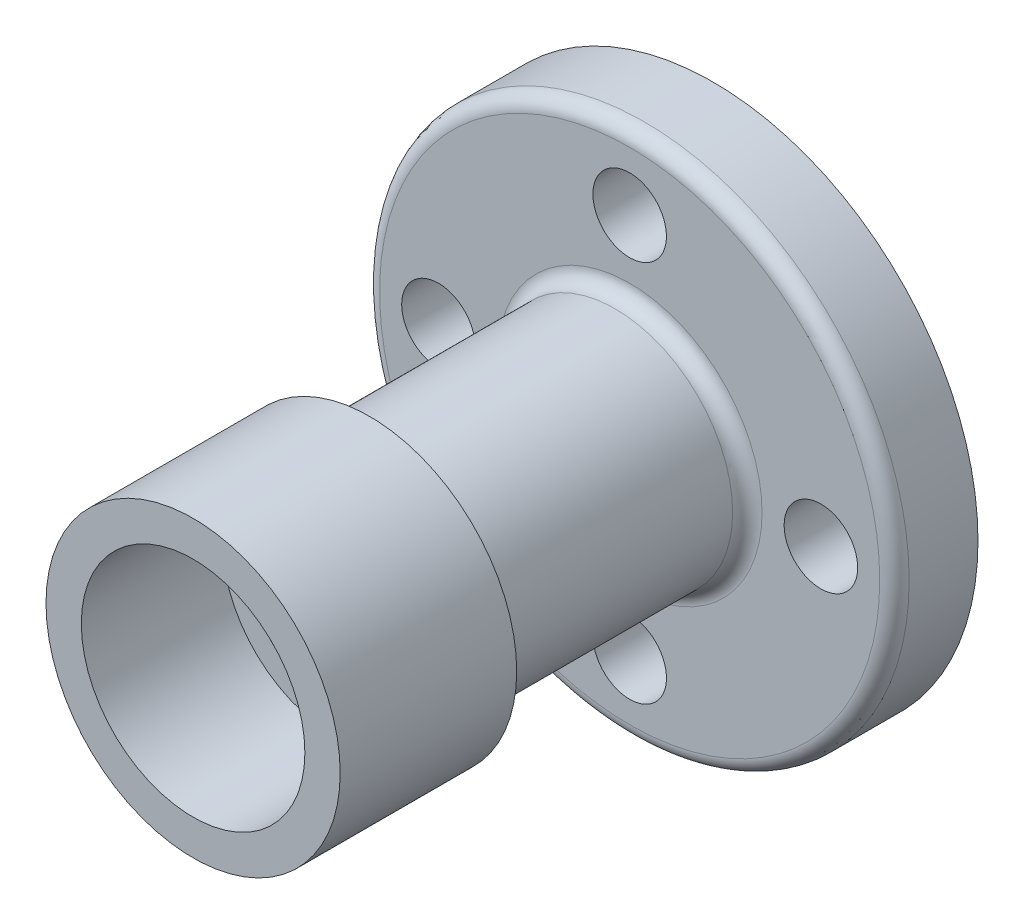
ISO-10303-21;
HEADER;
FILE_DESCRIPTION(('STEP AP214'),'2;1');
FILE_NAME('part.step','',(''),(''),'','','');
FILE_SCHEMA(('AUTOMOTIVE_DESIGN { 1 0 10303 214 1 1 1 1 }'));
ENDSEC;
DATA;
#1=APPLICATION_CONTEXT('core data for automotive mechanical design processes');
#2=APPLICATION_PROTOCOL_DEFINITION('international standard','automotive_design',2000,#1);
#3=PRODUCT_CONTEXT('',#1,'mechanical');
#4=PRODUCT('Part','Part','',(#3));
#5=PRODUCT_RELATED_PRODUCT_CATEGORY('part','',(#4));
#6=PRODUCT_DEFINITION_FORMATION('','',#4);
#7=PRODUCT_DEFINITION_CONTEXT('part definition',#1,'design');
#8=PRODUCT_DEFINITION('design','',#6,#7);
#9=PRODUCT_DEFINITION_SHAPE('','',#8);
#10=(LENGTH_UNIT() NAMED_UNIT(*) SI_UNIT(.MILLI.,.METRE.));
#11=(NAMED_UNIT(*) PLANE_ANGLE_UNIT() SI_UNIT($,.RADIAN.));
#12=(NAMED_UNIT(*) SI_UNIT($,.STERADIAN.) SOLID_ANGLE_UNIT());
#13=UNCERTAINTY_MEASURE_WITH_UNIT(LENGTH_MEASURE(1.E-05),#10,'distance_accuracy_value','');
#14=(GEOMETRIC_REPRESENTATION_CONTEXT(3) GLOBAL_UNCERTAINTY_ASSIGNED_CONTEXT((#13)) GLOBAL_UNIT_ASSIGNED_CONTEXT((#10,
#11,#12)) REPRESENTATION_CONTEXT('',''));
#15=CARTESIAN_POINT('',(0.,0.,0.));
#16=DIRECTION('',(0.,0.,1.));
#17=DIRECTION('',(1.,0.,0.));
#18=AXIS2_PLACEMENT_3D('',#15,#16,#17);
#19=CARTESIAN_POINT('',(0.,0.,64.4));
#20=DIRECTION('',(0.,0.,1.));
#21=DIRECTION('',(1.,0.,0.));
#22=AXIS2_PLACEMENT_3D('',#19,#20,#21);
#23=PLANE('',#22);
#24=CARTESIAN_POINT('',(0.,0.,64.4));
#25=DIRECTION('',(0.,0.,1.));
#26=DIRECTION('',(1.,0.,0.));
#27=AXIS2_PLACEMENT_3D('',#24,#25,#26);
#28=CIRCLE('',#27,15.);
#29=CARTESIAN_POINT('',(15.,0.,64.4));
#30=VERTEX_POINT('',#29);
#31=EDGE_CURVE('E102',#30,#30,#28,.T.);
#32=ORIENTED_EDGE('',*,*,#31,.F.);
#33=EDGE_LOOP('',(#32));
#34=FACE_BOUND('',#33,.T.);
#35=CARTESIAN_POINT('',(0.,0.,64.4));
#36=DIRECTION('',(0.,0.,1.));
#37=DIRECTION('',(1.,0.,0.));
#38=AXIS2_PLACEMENT_3D('',#35,#36,#37);
#39=CIRCLE('',#38,19.);
#40=CARTESIAN_POINT('',(19.,0.,64.4));
#41=VERTEX_POINT('',#40);
#42=EDGE_CURVE('E112',#41,#41,#39,.T.);
#43=ORIENTED_EDGE('',*,*,#42,.T.);
#44=EDGE_LOOP('',(#43));
#45=FACE_BOUND('',#44,.T.);
#46=ADVANCED_FACE('F44',(#34,#45),#23,.T.);
#47=CARTESIAN_POINT('',(0.,0.,14.2));
#48=DIRECTION('',(0.,0.,1.));
#49=DIRECTION('',(1.,0.,0.));
#50=AXIS2_PLACEMENT_3D('',#47,#48,#49);
#51=PLANE('',#50);
#52=CARTESIAN_POINT('',(0.,0.,14.2));
#53=DIRECTION('',(0.,0.,1.));
#54=DIRECTION('',(1.,0.,0.));
#55=AXIS2_PLACEMENT_3D('',#52,#53,#54);
#56=CIRCLE('',#55,22.5);
#57=CARTESIAN_POINT('',(22.5,0.,14.2));
#58=VERTEX_POINT('',#57);
#59=EDGE_CURVE('E11',#58,#58,#56,.F.);
#60=ORIENTED_EDGE('',*,*,#59,.T.);
#61=EDGE_LOOP('',(#60));
#62=FACE_BOUND('',#61,.T.);
#63=CARTESIAN_POINT('',(0.,0.,14.2));
#64=DIRECTION('',(0.,0.,1.));
#65=DIRECTION('',(1.,0.,0.));
#66=AXIS2_PLACEMENT_3D('',#63,#64,#65);
#67=CIRCLE('',#66,42.5);
#68=CARTESIAN_POINT('',(42.5,0.,14.2));
#69=VERTEX_POINT('',#68);
#70=EDGE_CURVE('E58',#69,#69,#67,.T.);
#71=ORIENTED_EDGE('',*,*,#70,.T.);
#72=EDGE_LOOP('',(#71));
#73=FACE_BOUND('',#72,.T.);
#74=CARTESIAN_POINT('',(0.,32.5,14.2));
#75=DIRECTION('',(0.,0.,-1.));
#76=DIRECTION('',(-1.,0.,0.));
#77=AXIS2_PLACEMENT_3D('',#74,#75,#76);
#78=CIRCLE('',#77,6.25);
#79=CARTESIAN_POINT('',(-6.25,32.5,14.2));
#80=VERTEX_POINT('',#79);
#81=EDGE_CURVE('E78',#80,#80,#78,.T.);
#82=ORIENTED_EDGE('',*,*,#81,.T.);
#83=EDGE_LOOP('',(#82));
#84=FACE_BOUND('',#83,.T.);
#85=CARTESIAN_POINT('',(0.,-32.5,14.2));
#86=DIRECTION('',(0.,0.,-1.));
#87=DIRECTION('',(-1.,0.,0.));
#88=AXIS2_PLACEMENT_3D('',#85,#86,#87);
#89=CIRCLE('',#88,6.25);
#90=CARTESIAN_POINT('',(-6.25000000000001,-32.5,14.2));
#91=VERTEX_POINT('',#90);
#92=EDGE_CURVE('E85',#91,#91,#89,.T.);
#93=ORIENTED_EDGE('',*,*,#92,.T.);
#94=EDGE_LOOP('',(#93));
#95=FACE_BOUND('',#94,.T.);
#96=CARTESIAN_POINT('',(-32.5,0.,14.2));
#97=DIRECTION('',(0.,0.,-1.));
#98=DIRECTION('',(-1.,0.,0.));
#99=AXIS2_PLACEMENT_3D('',#96,#97,#98);
#100=CIRCLE('',#99,6.25);
#101=CARTESIAN_POINT('',(-38.75,0.,14.2));
#102=VERTEX_POINT('',#101);
#103=EDGE_CURVE('E93',#102,#102,#100,.T.);
#104=ORIENTED_EDGE('',*,*,#103,.T.);
#105=EDGE_LOOP('',(#104));
#106=FACE_BOUND('',#105,.T.);
#107=CARTESIAN_POINT('',(32.5,0.,14.2));
#108=DIRECTION('',(0.,0.,-1.));
#109=DIRECTION('',(-1.,0.,0.));
#110=AXIS2_PLACEMENT_3D('',#107,#108,#109);
#111=CIRCLE('',#110,6.25);
#112=CARTESIAN_POINT('',(26.25,0.,14.2));
#113=VERTEX_POINT('',#112);
#114=EDGE_CURVE('E74',#113,#113,#111,.T.);
#115=ORIENTED_EDGE('',*,*,#114,.T.);
#116=EDGE_LOOP('',(#115));
#117=FACE_BOUND('',#116,.T.);
#118=ADVANCED_FACE('F131',(#62,#73,#84,#95,#106,#117),#51,.T.);
#119=CARTESIAN_POINT('',(0.,0.,0.));
#120=DIRECTION('',(0.,0.,1.));
#121=DIRECTION('',(1.,0.,0.));
#122=AXIS2_PLACEMENT_3D('',#119,#120,#121);
#123=PLANE('',#122);
#124=CARTESIAN_POINT('',(0.,0.,0.));
#125=DIRECTION('',(0.,0.,1.));
#126=DIRECTION('',(1.,0.,0.));
#127=AXIS2_PLACEMENT_3D('',#124,#125,#126);
#128=CIRCLE('',#127,18.5);
#129=CARTESIAN_POINT('',(18.5,0.,0.));
#130=VERTEX_POINT('',#129);
#131=EDGE_CURVE('E69',#130,#130,#128,.T.);
#132=ORIENTED_EDGE('',*,*,#131,.T.);
#133=EDGE_LOOP('',(#132));
#134=FACE_BOUND('',#133,.T.);
#135=CARTESIAN_POINT('',(32.5,0.,0.));
#136=DIRECTION('',(0.,0.,-1.));
#137=DIRECTION('',(-1.,0.,0.));
#138=AXIS2_PLACEMENT_3D('',#135,#136,#137);
#139=CIRCLE('',#138,6.25);
#140=CARTESIAN_POINT('',(26.25,0.,0.));
#141=VERTEX_POINT('',#140);
#142=EDGE_CURVE('E94',#141,#141,#139,.T.);
#143=ORIENTED_EDGE('',*,*,#142,.F.);
#144=EDGE_LOOP('',(#143));
#145=FACE_BOUND('',#144,.T.);
#146=CARTESIAN_POINT('',(-32.5,0.,0.));
#147=DIRECTION('',(0.,0.,-1.));
#148=DIRECTION('',(-1.,0.,0.));
#149=AXIS2_PLACEMENT_3D('',#146,#147,#148);
#150=CIRCLE('',#149,6.25);
#151=CARTESIAN_POINT('',(-38.75,0.,0.));
#152=VERTEX_POINT('',#151);
#153=EDGE_CURVE('E86',#152,#152,#150,.T.);
#154=ORIENTED_EDGE('',*,*,#153,.F.);
#155=EDGE_LOOP('',(#154));
#156=FACE_BOUND('',#155,.T.);
#157=CARTESIAN_POINT('',(0.,-32.5,0.));
#158=DIRECTION('',(0.,0.,-1.));
#159=DIRECTION('',(-1.,0.,0.));
#160=AXIS2_PLACEMENT_3D('',#157,#158,#159);
#161=CIRCLE('',#160,6.25);
#162=CARTESIAN_POINT('',(-6.25000000000001,-32.5,0.));
#163=VERTEX_POINT('',#162);
#164=EDGE_CURVE('E82',#163,#163,#161,.T.);
#165=ORIENTED_EDGE('',*,*,#164,.F.);
#166=EDGE_LOOP('',(#165));
#167=FACE_BOUND('',#166,.T.);
#168=CARTESIAN_POINT('',(0.,32.5,0.));
#169=DIRECTION('',(0.,0.,-1.));
#170=DIRECTION('',(-1.,0.,0.));
#171=AXIS2_PLACEMENT_3D('',#168,#169,#170);
#172=CIRCLE('',#171,6.25);
#173=CARTESIAN_POINT('',(-6.25,32.5,0.));
#174=VERTEX_POINT('',#173);
#175=EDGE_CURVE('E73',#174,#174,#172,.T.);
#176=ORIENTED_EDGE('',*,*,#175,.F.);
#177=EDGE_LOOP('',(#176));
#178=FACE_BOUND('',#177,.T.);
#179=CARTESIAN_POINT('',(0.,0.,0.));
#180=DIRECTION('',(0.,0.,1.));
#181=DIRECTION('',(1.,0.,0.));
#182=AXIS2_PLACEMENT_3D('',#179,#180,#181);
#183=CIRCLE('',#182,45.);
#184=CARTESIAN_POINT('',(45.,0.,0.));
#185=VERTEX_POINT('',#184);
#186=EDGE_CURVE('E72',#185,#185,#183,.T.);
#187=ORIENTED_EDGE('',*,*,#186,.F.);
#188=EDGE_LOOP('',(#187));
#189=FACE_BOUND('',#188,.T.);
#190=ADVANCED_FACE('F143',(#134,#145,#156,#167,#178,#189),#123,.F.);
#191=CARTESIAN_POINT('',(0.,0.,14.2));
#192=DIRECTION('',(0.,0.,-1.));
#193=DIRECTION('',(-1.,0.,0.));
#194=AXIS2_PLACEMENT_3D('',#191,#192,#193);
#195=CYLINDRICAL_SURFACE('',#194,45.);
#196=CARTESIAN_POINT('',(0.,0.,11.7));
#197=DIRECTION('',(0.,0.,1.));
#198=DIRECTION('',(1.,0.,0.));
#199=AXIS2_PLACEMENT_3D('',#196,#197,#198);
#200=CIRCLE('',#199,45.);
#201=CARTESIAN_POINT('',(45.,0.,11.7));
#202=VERTEX_POINT('',#201);
#203=EDGE_CURVE('E57',#202,#202,#200,.F.);
#204=ORIENTED_EDGE('',*,*,#203,.T.);
#205=EDGE_LOOP('',(#204));
#206=FACE_BOUND('',#205,.T.);
#207=ORIENTED_EDGE('',*,*,#186,.T.);
#208=EDGE_LOOP('',(#207));
#209=FACE_BOUND('',#208,.T.);
#210=ADVANCED_FACE('F172',(#206,#209),#195,.T.);
#211=CARTESIAN_POINT('',(0.,0.,14.2));
#212=DIRECTION('',(0.,0.,-1.));
#213=DIRECTION('',(-1.,0.,0.));
#214=AXIS2_PLACEMENT_3D('',#211,#212,#213);
#215=CYLINDRICAL_SURFACE('',#214,15.);
#216=CARTESIAN_POINT('',(0.,0.,3.));
#217=DIRECTION('',(0.,0.,1.));
#218=DIRECTION('',(1.,0.,0.));
#219=AXIS2_PLACEMENT_3D('',#216,#217,#218);
#220=CIRCLE('',#219,15.);
#221=CARTESIAN_POINT('',(15.,0.,3.));
#222=VERTEX_POINT('',#221);
#223=EDGE_CURVE('E61',#222,#222,#220,.F.);
#224=ORIENTED_EDGE('',*,*,#223,.T.);
#225=EDGE_LOOP('',(#224));
#226=FACE_BOUND('',#225,.T.);
#227=ORIENTED_EDGE('',*,*,#31,.T.);
#228=EDGE_LOOP('',(#227));
#229=FACE_BOUND('',#228,.T.);
#230=ADVANCED_FACE('F169',(#226,#229),#215,.F.);
#231=CARTESIAN_POINT('',(0.,32.5,14.2));
#232=DIRECTION('',(0.,0.,-1.));
#233=DIRECTION('',(-1.,0.,0.));
#234=AXIS2_PLACEMENT_3D('',#231,#232,#233);
#235=CYLINDRICAL_SURFACE('',#234,6.25);
#236=ORIENTED_EDGE('',*,*,#81,.F.);
#237=EDGE_LOOP('',(#236));
#238=FACE_BOUND('',#237,.T.);
#239=ORIENTED_EDGE('',*,*,#175,.T.);
#240=EDGE_LOOP('',(#239));
#241=FACE_BOUND('',#240,.T.);
#242=ADVANCED_FACE('F163',(#238,#241),#235,.F.);
#243=CARTESIAN_POINT('',(0.,-32.5,14.2));
#244=DIRECTION('',(0.,0.,-1.));
#245=DIRECTION('',(-1.,0.,0.));
#246=AXIS2_PLACEMENT_3D('',#243,#244,#245);
#247=CYLINDRICAL_SURFACE('',#246,6.25);
#248=ORIENTED_EDGE('',*,*,#92,.F.);
#249=EDGE_LOOP('',(#248));
#250=FACE_BOUND('',#249,.T.);
#251=ORIENTED_EDGE('',*,*,#164,.T.);
#252=EDGE_LOOP('',(#251));
#253=FACE_BOUND('',#252,.T.);
#254=ADVANCED_FACE('F159',(#250,#253),#247,.F.);
#255=CARTESIAN_POINT('',(-32.5,0.,14.2));
#256=DIRECTION('',(0.,0.,-1.));
#257=DIRECTION('',(-1.,0.,0.));
#258=AXIS2_PLACEMENT_3D('',#255,#256,#257);
#259=CYLINDRICAL_SURFACE('',#258,6.25);
#260=ORIENTED_EDGE('',*,*,#103,.F.);
#261=EDGE_LOOP('',(#260));
#262=FACE_BOUND('',#261,.T.);
#263=ORIENTED_EDGE('',*,*,#153,.T.);
#264=EDGE_LOOP('',(#263));
#265=FACE_BOUND('',#264,.T.);
#266=ADVANCED_FACE('F156',(#262,#265),#259,.F.);
#267=CARTESIAN_POINT('',(32.5,0.,14.2));
#268=DIRECTION('',(0.,0.,-1.));
#269=DIRECTION('',(-1.,0.,0.));
#270=AXIS2_PLACEMENT_3D('',#267,#268,#269);
#271=CYLINDRICAL_SURFACE('',#270,6.25);
#272=ORIENTED_EDGE('',*,*,#114,.F.);
#273=EDGE_LOOP('',(#272));
#274=FACE_BOUND('',#273,.T.);
#275=ORIENTED_EDGE('',*,*,#142,.T.);
#276=EDGE_LOOP('',(#275));
#277=FACE_BOUND('',#276,.T.);
#278=ADVANCED_FACE('F153',(#274,#277),#271,.F.);
#279=CARTESIAN_POINT('',(0.,0.,0.));
#280=DIRECTION('',(0.,0.,-1.));
#281=DIRECTION('',(-1.,0.,0.));
#282=AXIS2_PLACEMENT_3D('',#279,#280,#281);
#283=CONICAL_SURFACE('',#282,18.5,0.862170054667228);
#284=ORIENTED_EDGE('',*,*,#223,.F.);
#285=EDGE_LOOP('',(#284));
#286=FACE_BOUND('',#285,.T.);
#287=ORIENTED_EDGE('',*,*,#131,.F.);
#288=EDGE_LOOP('',(#287));
#289=FACE_BOUND('',#288,.T.);
#290=ADVANCED_FACE('F155',(#286,#289),#283,.F.);
#291=CARTESIAN_POINT('',(0.,0.,58.4));
#292=DIRECTION('',(0.,0.,-1.));
#293=DIRECTION('',(-1.,0.,0.));
#294=AXIS2_PLACEMENT_3D('',#291,#292,#293);
#295=CYLINDRICAL_SURFACE('',#294,20.);
#296=CARTESIAN_POINT('',(0.,0.,16.7));
#297=DIRECTION('',(0.,0.,1.));
#298=DIRECTION('',(1.,0.,0.));
#299=AXIS2_PLACEMENT_3D('',#296,#297,#298);
#300=CIRCLE('',#299,20.);
#301=CARTESIAN_POINT('',(20.,0.,16.7));
#302=VERTEX_POINT('',#301);
#303=EDGE_CURVE('E55',#302,#302,#300,.T.);
#304=ORIENTED_EDGE('',*,*,#303,.T.);
#305=EDGE_LOOP('',(#304));
#306=FACE_BOUND('',#305,.T.);
#307=CARTESIAN_POINT('',(0.,0.,58.4));
#308=DIRECTION('',(0.,0.,1.));
#309=DIRECTION('',(1.,0.,0.));
#310=AXIS2_PLACEMENT_3D('',#307,#308,#309);
#311=CIRCLE('',#310,20.);
#312=CARTESIAN_POINT('',(20.,0.,58.4));
#313=VERTEX_POINT('',#312);
#314=EDGE_CURVE('E79',#313,#313,#311,.T.);
#315=ORIENTED_EDGE('',*,*,#314,.F.);
#316=EDGE_LOOP('',(#315));
#317=FACE_BOUND('',#316,.T.);
#318=ADVANCED_FACE('F149',(#306,#317),#295,.T.);
#319=CARTESIAN_POINT('',(0.,0.,11.7));
#320=DIRECTION('',(0.,0.,1.));
#321=DIRECTION('',(1.,0.,0.));
#322=AXIS2_PLACEMENT_3D('',#319,#320,#321);
#323=TOROIDAL_SURFACE('',#322,42.5,2.5);
#324=ORIENTED_EDGE('',*,*,#203,.F.);
#325=EDGE_LOOP('',(#324));
#326=FACE_BOUND('',#325,.T.);
#327=ORIENTED_EDGE('',*,*,#70,.F.);
#328=EDGE_LOOP('',(#327));
#329=FACE_BOUND('',#328,.T.);
#330=ADVANCED_FACE('F148',(#326,#329),#323,.T.);
#331=CARTESIAN_POINT('',(0.,0.,58.4));
#332=DIRECTION('',(0.,0.,1.));
#333=DIRECTION('',(1.,0.,0.));
#334=AXIS2_PLACEMENT_3D('',#331,#332,#333);
#335=PLANE('',#334);
#336=ORIENTED_EDGE('',*,*,#314,.T.);
#337=EDGE_LOOP('',(#336));
#338=FACE_BOUND('',#337,.T.);
#339=CARTESIAN_POINT('',(0.,0.,58.4));
#340=DIRECTION('',(0.,0.,1.));
#341=DIRECTION('',(1.,0.,0.));
#342=AXIS2_PLACEMENT_3D('',#339,#340,#341);
#343=CIRCLE('',#342,25.);
#344=CARTESIAN_POINT('',(25.,0.,58.4));
#345=VERTEX_POINT('',#344);
#346=EDGE_CURVE('E101',#345,#345,#343,.T.);
#347=ORIENTED_EDGE('',*,*,#346,.F.);
#348=EDGE_LOOP('',(#347));
#349=FACE_BOUND('',#348,.T.);
#350=ADVANCED_FACE('F128',(#338,#349),#335,.F.);
#351=CARTESIAN_POINT('',(0.,0.,64.4));
#352=DIRECTION('',(0.,0.,-1.));
#353=DIRECTION('',(-1.,0.,0.));
#354=AXIS2_PLACEMENT_3D('',#351,#352,#353);
#355=CYLINDRICAL_SURFACE('',#354,25.);
#356=ORIENTED_EDGE('',*,*,#346,.T.);
#357=EDGE_LOOP('',(#356));
#358=FACE_BOUND('',#357,.T.);
#359=CARTESIAN_POINT('',(0.,0.,88.4));
#360=DIRECTION('',(0.,0.,1.));
#361=DIRECTION('',(1.,0.,0.));
#362=AXIS2_PLACEMENT_3D('',#359,#360,#361);
#363=CIRCLE('',#362,25.);
#364=CARTESIAN_POINT('',(25.,0.,88.4));
#365=VERTEX_POINT('',#364);
#366=EDGE_CURVE('E110',#365,#365,#363,.T.);
#367=ORIENTED_EDGE('',*,*,#366,.F.);
#368=EDGE_LOOP('',(#367));
#369=FACE_BOUND('',#368,.T.);
#370=ADVANCED_FACE('F122',(#358,#369),#355,.T.);
#371=CARTESIAN_POINT('',(0.,0.,88.4));
#372=DIRECTION('',(0.,0.,1.));
#373=DIRECTION('',(1.,0.,0.));
#374=AXIS2_PLACEMENT_3D('',#371,#372,#373);
#375=PLANE('',#374);
#376=ORIENTED_EDGE('',*,*,#366,.T.);
#377=EDGE_LOOP('',(#376));
#378=FACE_BOUND('',#377,.T.);
#379=CARTESIAN_POINT('',(0.,0.,88.4));
#380=DIRECTION('',(0.,0.,1.));
#381=DIRECTION('',(1.,0.,0.));
#382=AXIS2_PLACEMENT_3D('',#379,#380,#381);
#383=CIRCLE('',#382,19.);
#384=CARTESIAN_POINT('',(19.,0.,88.4));
#385=VERTEX_POINT('',#384);
#386=EDGE_CURVE('E109',#385,#385,#383,.T.);
#387=ORIENTED_EDGE('',*,*,#386,.F.);
#388=EDGE_LOOP('',(#387));
#389=FACE_BOUND('',#388,.T.);
#390=ADVANCED_FACE('F116',(#378,#389),#375,.T.);
#391=CARTESIAN_POINT('',(0.,0.,88.4));
#392=DIRECTION('',(0.,0.,-1.));
#393=DIRECTION('',(-1.,0.,0.));
#394=AXIS2_PLACEMENT_3D('',#391,#392,#393);
#395=CYLINDRICAL_SURFACE('',#394,19.);
#396=ORIENTED_EDGE('',*,*,#386,.T.);
#397=EDGE_LOOP('',(#396));
#398=FACE_BOUND('',#397,.T.);
#399=ORIENTED_EDGE('',*,*,#42,.F.);
#400=EDGE_LOOP('',(#399));
#401=FACE_BOUND('',#400,.T.);
#402=ADVANCED_FACE('F120',(#398,#401),#395,.F.);
#403=CARTESIAN_POINT('',(0.,0.,16.7));
#404=DIRECTION('',(0.,0.,1.));
#405=DIRECTION('',(1.,0.,0.));
#406=AXIS2_PLACEMENT_3D('',#403,#404,#405);
#407=TOROIDAL_SURFACE('',#406,22.5,2.5);
#408=ORIENTED_EDGE('',*,*,#59,.F.);
#409=EDGE_LOOP('',(#408));
#410=FACE_BOUND('',#409,.T.);
#411=ORIENTED_EDGE('',*,*,#303,.F.);
#412=EDGE_LOOP('',(#411));
#413=FACE_BOUND('',#412,.T.);
#414=ADVANCED_FACE('F50',(#410,#413),#407,.F.);
#415=CLOSED_SHELL('',(#46,#118,#190,#210,#230,#242,#254,#266,#278,#290,#318,#330,#350,#370,#390,
#402,#414));
#416=MANIFOLD_SOLID_BREP('B2',#415);
#417=ADVANCED_BREP_SHAPE_REPRESENTATION('',(#18,#416),#14);
#418=SHAPE_DEFINITION_REPRESENTATION(#9,#417);
ENDSEC;
END-ISO-10303-21;
